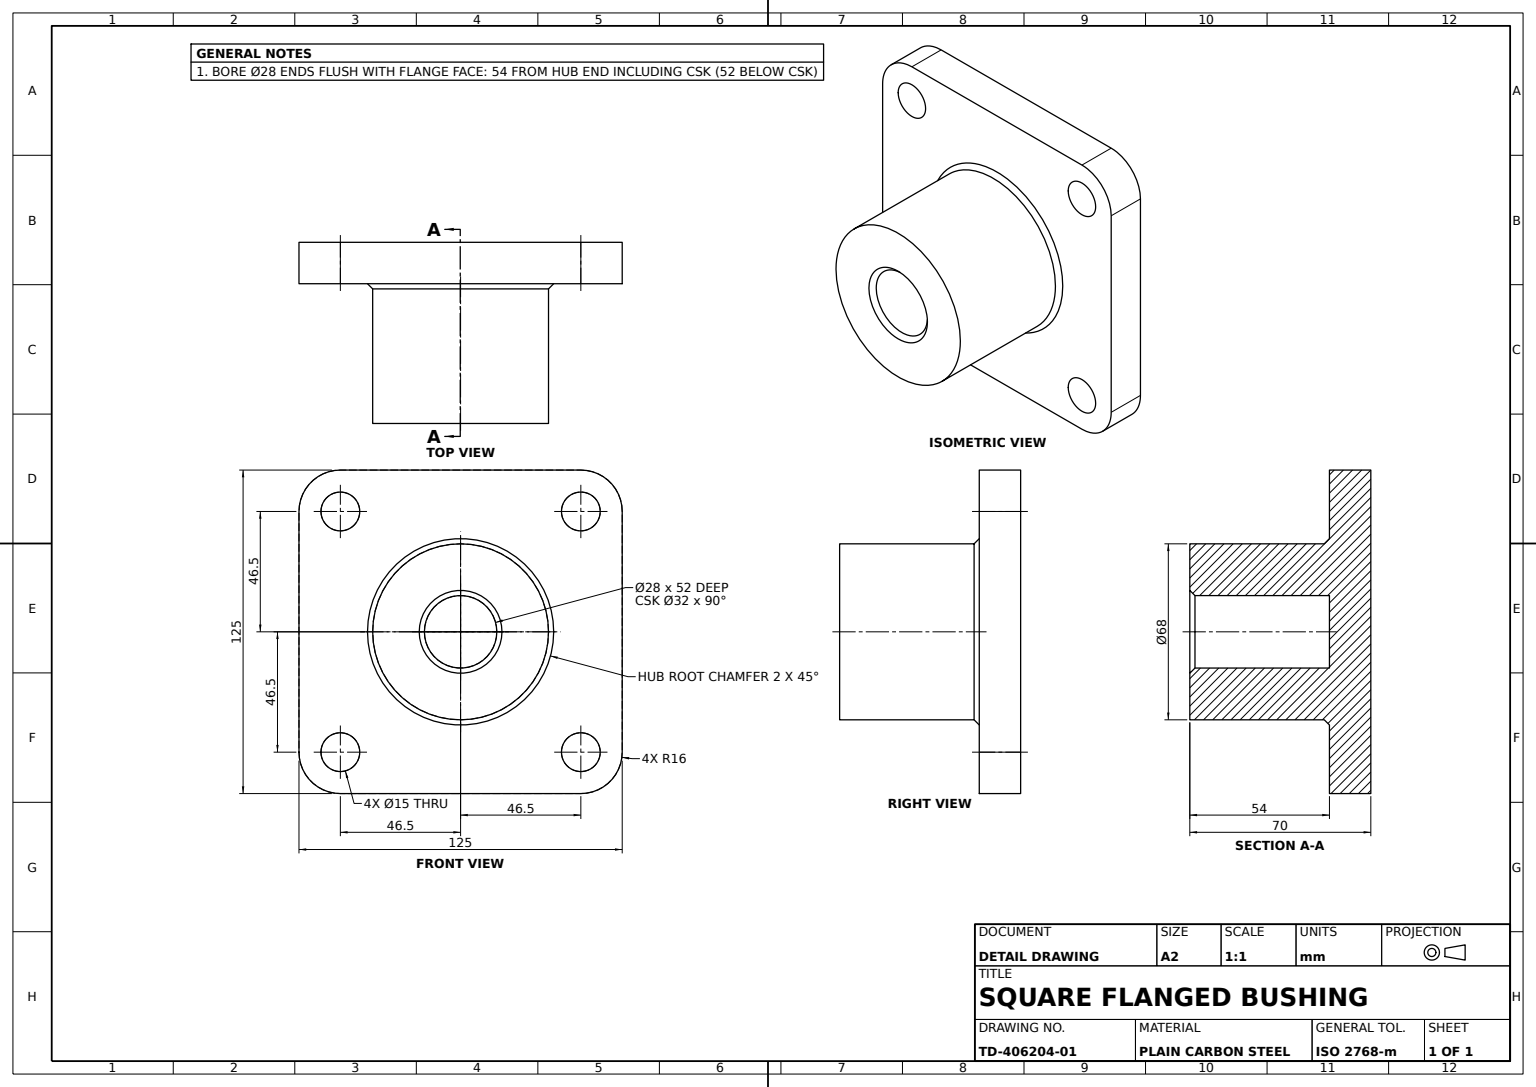
SolidWorks part; units mm, degrees
material "Plain Carbon Steel"
ref_plane "Front Plane" through (0, 0, 0) normal (0, 0, 1) x (1, 0, 0)
ref_plane "Top Plane" through (0, 0, 0) normal (0, 1, 0) x (1, 0, 0)
ref_plane "Right Plane" through (0, 0, 0) normal (1, 0, 0) x (0, 0, -1)
sketch "Flange Plate Sketch" plane through (0, 0, 0) normal (0, 0, 1) x (1, 0, 0)
  line L0 (16, 0) -> (109, 0)
  line L1 (125, -16) -> (125, -109)
  line L2 (109, -125) -> (16, -125)
  line L3 (0, -109) -> (0, -16)
  arc A0 (0, -109) -> (16, -125) centre (16, -109) ccw
  arc A1 (109, -125) -> (125, -109) centre (109, -109) ccw
  arc A2 (125, -16) -> (109, 0) centre (109, -16) ccw
  arc A3 (0, -16) -> (16, 0) centre (16, -16) cw
  point P13 (0, 0)
  dimension "D1" = 16
  dimension "D2" = 125
extrude "Flange Plate 125x125x16" add sketch "Flange Plate Sketch" along normal blind 16
sketch "Bolt Holes Sketch" plane through (0, 0, 16) normal (0, 0, 1) x (1, 0, 0)
  circle A0 centre (16, -16) radius 7.5
  circle A1 centre (109, -16) radius 7.5
  circle A2 centre (109, -109) radius 7.5
  circle A3 centre (16, -109) radius 7.5
  dimension "D1" = 15
  dimension "D2" = 15
  dimension "D3" = 15
  dimension "D4" = 15
  dimension "D5" = 15
extrude "Bolt Holes 4xØ15" cut sketch "Bolt Holes Sketch" against normal blind 16
sketch "Hub Sketch" plane through (0, 0, 16) normal (0, 0, 1) x (1, 0, 0)
  line L0 (16, -125) -> (109, -125) construction
  circle A0 centre (62.5, -62.5) radius 34
  dimension "D1" = 68
  dimension "D2" = 68
  dimension "D3" = 46.5
  dimension "D4" = 62.5
extrude "Hub Ø68x54" add sketch "Hub Sketch" along normal blind 54
chamfer "Hub Chamfer 2x45" distance 2 angle 45 1 edges at (96.5, -62.5, 16)
sketch "Bore Sketch" plane through (0, 0, 70) normal (0, 0, 1) x (1, 0, 0)
  circle A0 centre (62.5, -62.5) radius 14
  dimension "D1" = 28
  dimension "D2" = 28
extrude "Bore Ø28" cut sketch "Bore Sketch" against normal blind 54
chamfer "Bore Chamfer 2x45" distance 2 angle 45 1 edges at (76.5, -62.5, 70)
